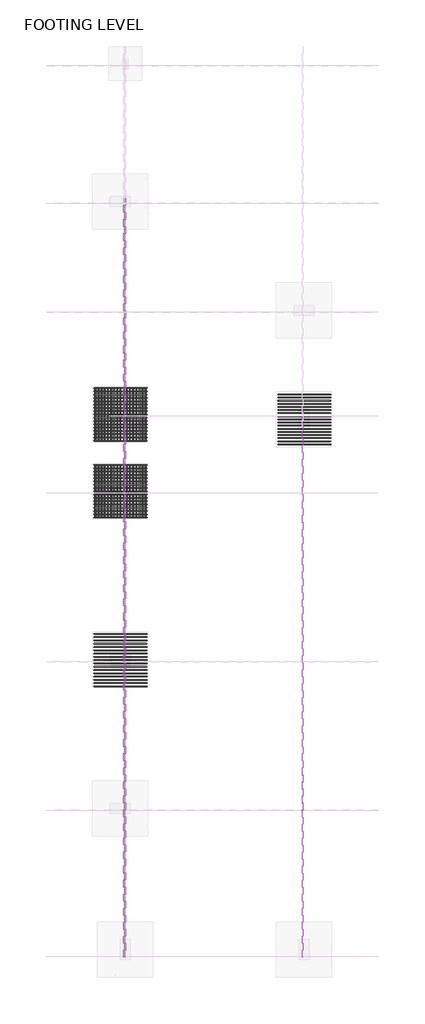
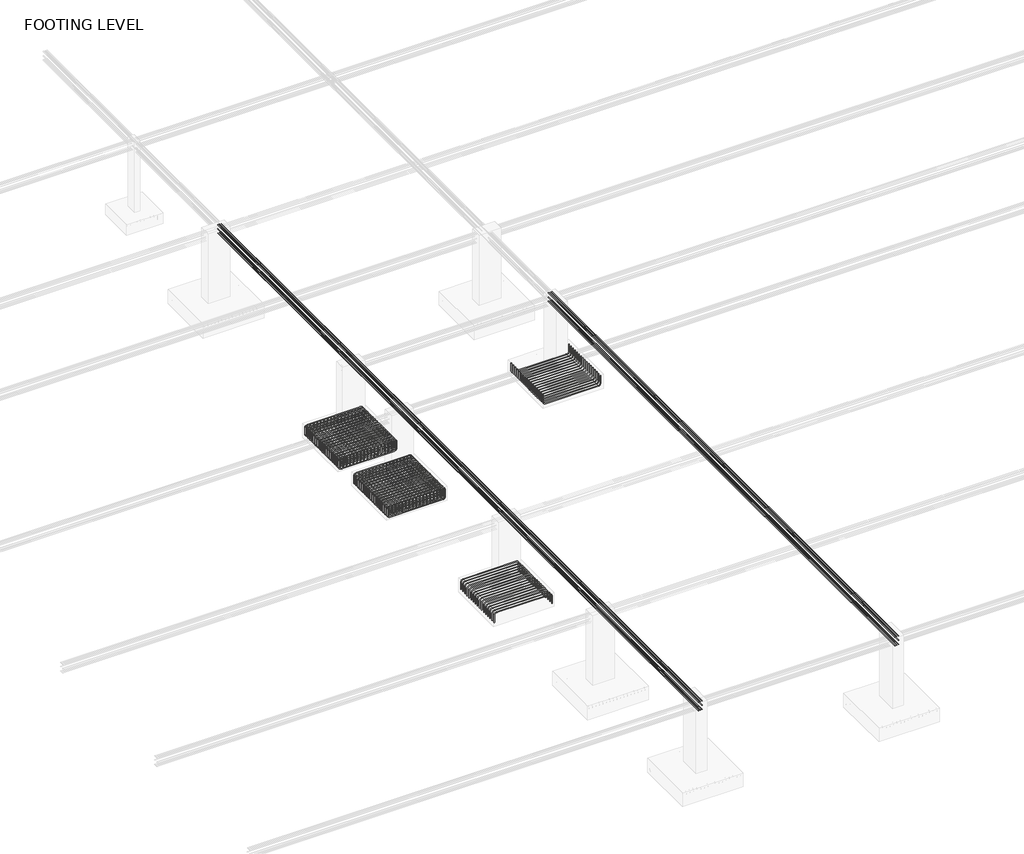
# One storey, part 7 of 19: 16 reinforcing bars.
"""IFC4 building model written with IfcOpenShell, lengths in millimetres."""

from ifc_helpers import new_model, si_unit, point, frame, origin, place, context, project, spatial, polyline, circle_curve, trimmed, segment, composite_curve, source, transform, mapped, element, save
from ifc_brep_helpers import swept_disk

model = new_model("IFC4")

# Units and contexts
model_context = context("Model", 3, world=origin())
ifc_project = project(units=[si_unit("LENGTHUNIT", "METRE", prefix="MILLI")], contexts=[model_context])

# Site, building, storey
site = spatial("IfcSite", under=ifc_project)
building = spatial("IfcBuilding", under=site)
storey = spatial("IfcBuildingStorey", under=building, Name="FOOTING LEVEL", Elevation=-3048.0)

# Reinforcing bars
placement = place(None, origin())
reinforcing_bar_shape = source(origin(), model_context, "Body", "SolidModel", [
    swept_disk(composite_curve([segment(polyline([(10639.8587563, -5025.9516566, -3148.0), (10639.8587563, -5025.9516566, -3470.1)]), True, "CONTINUOUS"), segment(trimmed(circle_curve(frame((10549.6587563, -5025.9516566, -3470.1), z_axis=(0.0, 1.0, 0.0), x_axis=(90.20000000000073, 0.0, 0.0)), 90.2), [point((10639.8587563, -5025.9516566, -3470.1))], [point((10549.6587563, -5025.9516566, -3560.3))], True, "CARTESIAN"), True, "CONTINUOUS"), segment(polyline([(10549.6587563, -5025.9516566, -3560.3), (8355.4587563, -5025.9516566, -3560.3)]), True, "CONTINUOUS"), segment(trimmed(circle_curve(frame((8355.4587563, -5025.9516566, -3470.1), z_axis=(0.0, 1.0, 0.0), x_axis=(0.0, 0.0, -90.20000000000027)), 90.2), [point((8355.4587563, -5025.9516566, -3560.3))], [point((8265.2587563, -5025.9516566, -3470.1))], True, "CARTESIAN"), True, "CONTINUOUS"), segment(polyline([(8265.2587563, -5025.9516566, -3470.1), (8265.2587563, -5025.9516566, -3148.0)]), True, "CONTINUOUS")], self_intersect=False), 12.7),
])
element("IfcReinforcingBar", 1, at=placement, inside=storey, context=model_context, shape_type="MappedRepresentation", body=[
    mapped(reinforcing_bar_shape, transform((0.0, 0.0, 0.0), x_axis=(1.0, 0.0, 0.0), y_axis=(0.0, 1.0, 0.0), z_axis=(0.0, 0.0, 1.0))),
    mapped(reinforcing_bar_shape, transform((0.0, 140.8090411, 0.0), x_axis=(1.0, 0.0, 0.0), y_axis=(0.0, 1.0, 0.0), z_axis=(0.0, 0.0, 1.0))),
    mapped(reinforcing_bar_shape, transform((0.0, 281.6180821, 0.0), x_axis=(1.0, 0.0, 0.0), y_axis=(0.0, 1.0, 0.0), z_axis=(0.0, 0.0, 1.0))),
    mapped(reinforcing_bar_shape, transform((0.0, 422.4271232, 0.0), x_axis=(1.0, 0.0, 0.0), y_axis=(0.0, 1.0, 0.0), z_axis=(0.0, 0.0, 1.0))),
    mapped(reinforcing_bar_shape, transform((0.0, 563.2361643, 0.0), x_axis=(1.0, 0.0, 0.0), y_axis=(0.0, 1.0, 0.0), z_axis=(0.0, 0.0, 1.0))),
    mapped(reinforcing_bar_shape, transform((0.0, 704.0452054, 0.0), x_axis=(1.0, 0.0, 0.0), y_axis=(0.0, 1.0, 0.0), z_axis=(0.0, 0.0, 1.0))),
    mapped(reinforcing_bar_shape, transform((0.0, 844.8542464, 0.0), x_axis=(1.0, 0.0, 0.0), y_axis=(0.0, 1.0, 0.0), z_axis=(0.0, 0.0, 1.0))),
    mapped(reinforcing_bar_shape, transform((0.0, 985.6632875, 0.0), x_axis=(1.0, 0.0, 0.0), y_axis=(0.0, 1.0, 0.0), z_axis=(0.0, 0.0, 1.0))),
    mapped(reinforcing_bar_shape, transform((0.0, 1126.4723286, 0.0), x_axis=(1.0, 0.0, 0.0), y_axis=(0.0, 1.0, 0.0), z_axis=(0.0, 0.0, 1.0))),
    mapped(reinforcing_bar_shape, transform((0.0, 1267.2813697, 0.0), x_axis=(1.0, 0.0, 0.0), y_axis=(0.0, 1.0, 0.0), z_axis=(0.0, 0.0, 1.0))),
    mapped(reinforcing_bar_shape, transform((0.0, 1408.0904107, 0.0), x_axis=(1.0, 0.0, 0.0), y_axis=(0.0, 1.0, 0.0), z_axis=(0.0, 0.0, 1.0))),
    mapped(reinforcing_bar_shape, transform((0.0, 1548.8994518, 0.0), x_axis=(1.0, 0.0, 0.0), y_axis=(0.0, 1.0, 0.0), z_axis=(0.0, 0.0, 1.0))),
    mapped(reinforcing_bar_shape, transform((0.0, 1689.7084929, 0.0), x_axis=(1.0, 0.0, 0.0), y_axis=(0.0, 1.0, 0.0), z_axis=(0.0, 0.0, 1.0))),
    mapped(reinforcing_bar_shape, transform((0.0, 1830.517534, 0.0), x_axis=(1.0, 0.0, 0.0), y_axis=(0.0, 1.0, 0.0), z_axis=(0.0, 0.0, 1.0))),
    mapped(reinforcing_bar_shape, transform((0.0, 1971.326575, 0.0), x_axis=(1.0, 0.0, 0.0), y_axis=(0.0, 1.0, 0.0), z_axis=(0.0, 0.0, 1.0))),
    mapped(reinforcing_bar_shape, transform((0.0, 2112.1356161, 0.0), x_axis=(1.0, 0.0, 0.0), y_axis=(0.0, 1.0, 0.0), z_axis=(0.0, 0.0, 1.0))),
    mapped(reinforcing_bar_shape, transform((0.0, 2252.9446572, 0.0), x_axis=(1.0, 0.0, 0.0), y_axis=(0.0, 1.0, 0.0), z_axis=(0.0, 0.0, 1.0))),
])
reinforcing_bar_2_shape = source(origin(), model_context, "Body", "SolidModel", [
    swept_disk(composite_curve([segment(polyline([(2334.0587563, -13575.4205555, -3523.0), (2334.0587563, -13575.4205555, -3200.9)]), True, "CONTINUOUS"), segment(trimmed(circle_curve(frame((2243.8587563, -13575.4205555, -3200.9), z_axis=(0.0, -1.0, 0.0), x_axis=(90.19999999999982, 0.0, 0.0)), 90.2), [point((2334.0587563, -13575.4205555, -3200.9))], [point((2243.8587563, -13575.4205555, -3110.7))], True, "CARTESIAN"), True, "CONTINUOUS"), segment(polyline([(2243.8587563, -13575.4205555, -3110.7), (49.6587563, -13575.4205555, -3110.7)]), True, "CONTINUOUS"), segment(trimmed(circle_curve(frame((49.6587563, -13575.4205555, -3200.9), z_axis=(0.0, -1.0, 0.0), x_axis=(0.0, 0.0, 90.20000000000027)), 90.2), [point((49.6587563, -13575.4205555, -3110.7))], [point((-40.5412437, -13575.4205555, -3200.9))], True, "CARTESIAN"), True, "CONTINUOUS"), segment(polyline([(-40.5412437, -13575.4205555, -3200.9), (-40.5412437, -13575.4205555, -3523.0)]), True, "CONTINUOUS")], self_intersect=False), 12.7),
])
element("IfcReinforcingBar", 2, at=placement, inside=storey, context=model_context, shape_type="MappedRepresentation", body=[
    mapped(reinforcing_bar_2_shape, transform((0.0, 0.0, 0.0), x_axis=(1.0, 0.0, 0.0), y_axis=(0.0, 1.0, 0.0), z_axis=(0.0, 0.0, 1.0))),
    mapped(reinforcing_bar_2_shape, transform((0.0, -148.4125, 0.0), x_axis=(1.0, 0.0, 0.0), y_axis=(0.0, 1.0, 0.0), z_axis=(0.0, 0.0, 1.0))),
    mapped(reinforcing_bar_2_shape, transform((0.0, -296.825, 0.0), x_axis=(1.0, 0.0, 0.0), y_axis=(0.0, 1.0, 0.0), z_axis=(0.0, 0.0, 1.0))),
    mapped(reinforcing_bar_2_shape, transform((0.0, -445.2375, 0.0), x_axis=(1.0, 0.0, 0.0), y_axis=(0.0, 1.0, 0.0), z_axis=(0.0, 0.0, 1.0))),
    mapped(reinforcing_bar_2_shape, transform((0.0, -593.65, 0.0), x_axis=(1.0, 0.0, 0.0), y_axis=(0.0, 1.0, 0.0), z_axis=(0.0, 0.0, 1.0))),
    mapped(reinforcing_bar_2_shape, transform((0.0, -742.0625, 0.0), x_axis=(1.0, 0.0, 0.0), y_axis=(0.0, 1.0, 0.0), z_axis=(0.0, 0.0, 1.0))),
    mapped(reinforcing_bar_2_shape, transform((0.0, -890.475, 0.0), x_axis=(1.0, 0.0, 0.0), y_axis=(0.0, 1.0, 0.0), z_axis=(0.0, 0.0, 1.0))),
    mapped(reinforcing_bar_2_shape, transform((0.0, -1038.8875, 0.0), x_axis=(1.0, 0.0, 0.0), y_axis=(0.0, 1.0, 0.0), z_axis=(0.0, 0.0, 1.0))),
    mapped(reinforcing_bar_2_shape, transform((0.0, -1187.3, 0.0), x_axis=(1.0, 0.0, 0.0), y_axis=(0.0, 1.0, 0.0), z_axis=(0.0, 0.0, 1.0))),
    mapped(reinforcing_bar_2_shape, transform((0.0, -1335.7125, 0.0), x_axis=(1.0, 0.0, 0.0), y_axis=(0.0, 1.0, 0.0), z_axis=(0.0, 0.0, 1.0))),
    mapped(reinforcing_bar_2_shape, transform((0.0, -1484.125, 0.0), x_axis=(1.0, 0.0, 0.0), y_axis=(0.0, 1.0, 0.0), z_axis=(0.0, 0.0, 1.0))),
    mapped(reinforcing_bar_2_shape, transform((0.0, -1632.5375, 0.0), x_axis=(1.0, 0.0, 0.0), y_axis=(0.0, 1.0, 0.0), z_axis=(0.0, 0.0, 1.0))),
    mapped(reinforcing_bar_2_shape, transform((0.0, -1780.95, 0.0), x_axis=(1.0, 0.0, 0.0), y_axis=(0.0, 1.0, 0.0), z_axis=(0.0, 0.0, 1.0))),
    mapped(reinforcing_bar_2_shape, transform((0.0, -1929.3625, 0.0), x_axis=(1.0, 0.0, 0.0), y_axis=(0.0, 1.0, 0.0), z_axis=(0.0, 0.0, 1.0))),
    mapped(reinforcing_bar_2_shape, transform((0.0, -2077.775, 0.0), x_axis=(1.0, 0.0, 0.0), y_axis=(0.0, 1.0, 0.0), z_axis=(0.0, 0.0, 1.0))),
    mapped(reinforcing_bar_2_shape, transform((0.0, -2226.1875, 0.0), x_axis=(1.0, 0.0, 0.0), y_axis=(0.0, 1.0, 0.0), z_axis=(0.0, 0.0, 1.0))),
    mapped(reinforcing_bar_2_shape, transform((0.0, -2374.6, 0.0), x_axis=(1.0, 0.0, 0.0), y_axis=(0.0, 1.0, 0.0), z_axis=(0.0, 0.0, 1.0))),
])
reinforcing_bar_3_shape = source(origin(), model_context, "Body", "SolidModel", [
    swept_disk(composite_curve([segment(polyline([(25.0276552, -8330.0205555, -3148.0), (25.0276552, -8330.0205555, -3470.1)]), True, "CONTINUOUS"), segment(trimmed(circle_curve(frame((25.0276552, -8239.8205555, -3470.1), z_axis=(1.0, 0.0, 0.0), x_axis=(0.0, -90.19999999999891, 0.0)), 90.2), [point((25.0276552, -8330.0205555, -3470.1))], [point((25.0276552, -8239.8205555, -3560.3))], True, "CARTESIAN"), True, "CONTINUOUS"), segment(polyline([(25.0276552, -8239.8205555, -3560.3), (25.0276552, -6045.6205555, -3560.3)]), True, "CONTINUOUS"), segment(trimmed(circle_curve(frame((25.0276552, -6045.6205555, -3470.1), z_axis=(1.0, 0.0, 0.0), x_axis=(0.0, 0.0, -90.20000000000027)), 90.2), [point((25.0276552, -6045.6205555, -3560.3))], [point((25.0276552, -5955.4205555, -3470.1))], True, "CARTESIAN"), True, "CONTINUOUS"), segment(polyline([(25.0276552, -5955.4205555, -3470.1), (25.0276552, -5955.4205555, -3148.0)]), True, "CONTINUOUS")], self_intersect=False), 12.7),
])
element("IfcReinforcingBar", 3, at=placement, inside=storey, context=model_context, shape_type="MappedRepresentation", body=[
    mapped(reinforcing_bar_3_shape, transform((0.0, 0.0, 0.0), x_axis=(1.0, 0.0, 0.0), y_axis=(0.0, 1.0, 0.0), z_axis=(0.0, 0.0, 1.0))),
    mapped(reinforcing_bar_3_shape, transform((140.8090411, 0.0, 0.0), x_axis=(1.0, 0.0, 0.0), y_axis=(0.0, 1.0, 0.0), z_axis=(0.0, 0.0, 1.0))),
    mapped(reinforcing_bar_3_shape, transform((281.6180821, 0.0, 0.0), x_axis=(1.0, 0.0, 0.0), y_axis=(0.0, 1.0, 0.0), z_axis=(0.0, 0.0, 1.0))),
    mapped(reinforcing_bar_3_shape, transform((422.4271232, 0.0, 0.0), x_axis=(1.0, 0.0, 0.0), y_axis=(0.0, 1.0, 0.0), z_axis=(0.0, 0.0, 1.0))),
    mapped(reinforcing_bar_3_shape, transform((563.2361643, 0.0, 0.0), x_axis=(1.0, 0.0, 0.0), y_axis=(0.0, 1.0, 0.0), z_axis=(0.0, 0.0, 1.0))),
    mapped(reinforcing_bar_3_shape, transform((704.0452054, 0.0, 0.0), x_axis=(1.0, 0.0, 0.0), y_axis=(0.0, 1.0, 0.0), z_axis=(0.0, 0.0, 1.0))),
    mapped(reinforcing_bar_3_shape, transform((844.8542464, 0.0, 0.0), x_axis=(1.0, 0.0, 0.0), y_axis=(0.0, 1.0, 0.0), z_axis=(0.0, 0.0, 1.0))),
    mapped(reinforcing_bar_3_shape, transform((985.6632875, 0.0, 0.0), x_axis=(1.0, 0.0, 0.0), y_axis=(0.0, 1.0, 0.0), z_axis=(0.0, 0.0, 1.0))),
    mapped(reinforcing_bar_3_shape, transform((1126.4723286, 0.0, 0.0), x_axis=(1.0, 0.0, 0.0), y_axis=(0.0, 1.0, 0.0), z_axis=(0.0, 0.0, 1.0))),
    mapped(reinforcing_bar_3_shape, transform((1267.2813697, 0.0, 0.0), x_axis=(1.0, 0.0, 0.0), y_axis=(0.0, 1.0, 0.0), z_axis=(0.0, 0.0, 1.0))),
    mapped(reinforcing_bar_3_shape, transform((1408.0904107, 0.0, 0.0), x_axis=(1.0, 0.0, 0.0), y_axis=(0.0, 1.0, 0.0), z_axis=(0.0, 0.0, 1.0))),
    mapped(reinforcing_bar_3_shape, transform((1548.8994518, 0.0, 0.0), x_axis=(1.0, 0.0, 0.0), y_axis=(0.0, 1.0, 0.0), z_axis=(0.0, 0.0, 1.0))),
    mapped(reinforcing_bar_3_shape, transform((1689.7084929, 0.0, 0.0), x_axis=(1.0, 0.0, 0.0), y_axis=(0.0, 1.0, 0.0), z_axis=(0.0, 0.0, 1.0))),
    mapped(reinforcing_bar_3_shape, transform((1830.517534, 0.0, 0.0), x_axis=(1.0, 0.0, 0.0), y_axis=(0.0, 1.0, 0.0), z_axis=(0.0, 0.0, 1.0))),
    mapped(reinforcing_bar_3_shape, transform((1971.326575, 0.0, 0.0), x_axis=(1.0, 0.0, 0.0), y_axis=(0.0, 1.0, 0.0), z_axis=(0.0, 0.0, 1.0))),
    mapped(reinforcing_bar_3_shape, transform((2112.1356161, 0.0, 0.0), x_axis=(1.0, 0.0, 0.0), y_axis=(0.0, 1.0, 0.0), z_axis=(0.0, 0.0, 1.0))),
    mapped(reinforcing_bar_3_shape, transform((2252.9446572, 0.0, 0.0), x_axis=(1.0, 0.0, 0.0), y_axis=(0.0, 1.0, 0.0), z_axis=(0.0, 0.0, 1.0))),
])
reinforcing_bar_4_shape = source(origin(), model_context, "Body", "SolidModel", [
    swept_disk(composite_curve([segment(polyline([(2300.4197045, -8330.0205555, -3548.0), (2300.4197045, -8330.0205555, -3225.9)]), True, "CONTINUOUS"), segment(trimmed(circle_curve(frame((2300.4197045, -8239.8205555, -3225.9), z_axis=(-1.0, 0.0, 0.0), x_axis=(0.0, -90.19999999999891, 0.0)), 90.2), [point((2300.4197045, -8330.0205555, -3225.9))], [point((2300.4197045, -8239.8205555, -3135.7))], True, "CARTESIAN"), True, "CONTINUOUS"), segment(polyline([(2300.4197045, -8239.8205555, -3135.7), (2300.4197045, -6045.6205555, -3135.7)]), True, "CONTINUOUS"), segment(trimmed(circle_curve(frame((2300.4197045, -6045.6205555, -3225.9), z_axis=(-1.0, 0.0, 0.0), x_axis=(0.0, 0.0, 90.20000000000027)), 90.2), [point((2300.4197045, -6045.6205555, -3135.7))], [point((2300.4197045, -5955.4205555, -3225.9))], True, "CARTESIAN"), True, "CONTINUOUS"), segment(polyline([(2300.4197045, -5955.4205555, -3225.9), (2300.4197045, -5955.4205555, -3548.0)]), True, "CONTINUOUS")], self_intersect=False), 12.7),
])
element("IfcReinforcingBar", 4, at=placement, inside=storey, context=model_context, shape_type="MappedRepresentation", body=[
    mapped(reinforcing_bar_4_shape, transform((0.0, 0.0, 0.0), x_axis=(1.0, 0.0, 0.0), y_axis=(0.0, 1.0, 0.0), z_axis=(0.0, 0.0, 1.0))),
    mapped(reinforcing_bar_4_shape, transform((-143.8496077, 0.0, 0.0), x_axis=(1.0, 0.0, 0.0), y_axis=(0.0, 1.0, 0.0), z_axis=(0.0, 0.0, 1.0))),
    mapped(reinforcing_bar_4_shape, transform((-287.6992155, 0.0, 0.0), x_axis=(1.0, 0.0, 0.0), y_axis=(0.0, 1.0, 0.0), z_axis=(0.0, 0.0, 1.0))),
    mapped(reinforcing_bar_4_shape, transform((-431.5488232, 0.0, 0.0), x_axis=(1.0, 0.0, 0.0), y_axis=(0.0, 1.0, 0.0), z_axis=(0.0, 0.0, 1.0))),
    mapped(reinforcing_bar_4_shape, transform((-575.398431, 0.0, 0.0), x_axis=(1.0, 0.0, 0.0), y_axis=(0.0, 1.0, 0.0), z_axis=(0.0, 0.0, 1.0))),
    mapped(reinforcing_bar_4_shape, transform((-719.2480387, 0.0, 0.0), x_axis=(1.0, 0.0, 0.0), y_axis=(0.0, 1.0, 0.0), z_axis=(0.0, 0.0, 1.0))),
    mapped(reinforcing_bar_4_shape, transform((-863.0976465, 0.0, 0.0), x_axis=(1.0, 0.0, 0.0), y_axis=(0.0, 1.0, 0.0), z_axis=(0.0, 0.0, 1.0))),
    mapped(reinforcing_bar_4_shape, transform((-1006.9472542, 0.0, 0.0), x_axis=(1.0, 0.0, 0.0), y_axis=(0.0, 1.0, 0.0), z_axis=(0.0, 0.0, 1.0))),
    mapped(reinforcing_bar_4_shape, transform((-1150.796862, 0.0, 0.0), x_axis=(1.0, 0.0, 0.0), y_axis=(0.0, 1.0, 0.0), z_axis=(0.0, 0.0, 1.0))),
    mapped(reinforcing_bar_4_shape, transform((-1294.6464697, 0.0, 0.0), x_axis=(1.0, 0.0, 0.0), y_axis=(0.0, 1.0, 0.0), z_axis=(0.0, 0.0, 1.0))),
    mapped(reinforcing_bar_4_shape, transform((-1438.4960775, 0.0, 0.0), x_axis=(1.0, 0.0, 0.0), y_axis=(0.0, 1.0, 0.0), z_axis=(0.0, 0.0, 1.0))),
    mapped(reinforcing_bar_4_shape, transform((-1582.3456852, 0.0, 0.0), x_axis=(1.0, 0.0, 0.0), y_axis=(0.0, 1.0, 0.0), z_axis=(0.0, 0.0, 1.0))),
    mapped(reinforcing_bar_4_shape, transform((-1726.195293, 0.0, 0.0), x_axis=(1.0, 0.0, 0.0), y_axis=(0.0, 1.0, 0.0), z_axis=(0.0, 0.0, 1.0))),
    mapped(reinforcing_bar_4_shape, transform((-1870.0449007, 0.0, 0.0), x_axis=(1.0, 0.0, 0.0), y_axis=(0.0, 1.0, 0.0), z_axis=(0.0, 0.0, 1.0))),
    mapped(reinforcing_bar_4_shape, transform((-2013.8945085, 0.0, 0.0), x_axis=(1.0, 0.0, 0.0), y_axis=(0.0, 1.0, 0.0), z_axis=(0.0, 0.0, 1.0))),
    mapped(reinforcing_bar_4_shape, transform((-2157.7441162, 0.0, 0.0), x_axis=(1.0, 0.0, 0.0), y_axis=(0.0, 1.0, 0.0), z_axis=(0.0, 0.0, 1.0))),
    mapped(reinforcing_bar_4_shape, transform((-2301.5937239, 0.0, 0.0), x_axis=(1.0, 0.0, 0.0), y_axis=(0.0, 1.0, 0.0), z_axis=(0.0, 0.0, 1.0))),
])
reinforcing_bar_5_shape = source(origin(), model_context, "Body", "SolidModel", [
    swept_disk(composite_curve([segment(polyline([(-40.5412437, -5955.4205555, -3173.0), (-40.5412437, -5955.4205555, -3495.1)]), True, "CONTINUOUS"), segment(trimmed(circle_curve(frame((49.6587563, -5955.4205555, -3495.1), z_axis=(0.0, -1.0, 0.0), x_axis=(-90.2, 0.0, 0.0)), 90.2), [point((-40.5412437, -5955.4205555, -3495.1))], [point((49.6587563, -5955.4205555, -3585.3))], True, "CARTESIAN"), True, "CONTINUOUS"), segment(polyline([(49.6587563, -5955.4205555, -3585.3), (2243.8587563, -5955.4205555, -3585.3)]), True, "CONTINUOUS"), segment(trimmed(circle_curve(frame((2243.8587563, -5955.4205555, -3495.1), z_axis=(0.0, -1.0, 0.0), x_axis=(0.0, 0.0, -90.20000000000027)), 90.2), [point((2243.8587563, -5955.4205555, -3585.3))], [point((2334.0587563, -5955.4205555, -3495.1))], True, "CARTESIAN"), True, "CONTINUOUS"), segment(polyline([(2334.0587563, -5955.4205555, -3495.1), (2334.0587563, -5955.4205555, -3173.0)]), True, "CONTINUOUS")], self_intersect=False), 12.7),
])
element("IfcReinforcingBar", 5, at=placement, inside=storey, context=model_context, shape_type="MappedRepresentation", body=[
    mapped(reinforcing_bar_5_shape, transform((0.0, 0.0, 0.0), x_axis=(1.0, 0.0, 0.0), y_axis=(0.0, 1.0, 0.0), z_axis=(0.0, 0.0, 1.0))),
    mapped(reinforcing_bar_5_shape, transform((0.0, -148.4125, 0.0), x_axis=(1.0, 0.0, 0.0), y_axis=(0.0, 1.0, 0.0), z_axis=(0.0, 0.0, 1.0))),
    mapped(reinforcing_bar_5_shape, transform((0.0, -296.825, 0.0), x_axis=(1.0, 0.0, 0.0), y_axis=(0.0, 1.0, 0.0), z_axis=(0.0, 0.0, 1.0))),
    mapped(reinforcing_bar_5_shape, transform((0.0, -445.2375, 0.0), x_axis=(1.0, 0.0, 0.0), y_axis=(0.0, 1.0, 0.0), z_axis=(0.0, 0.0, 1.0))),
    mapped(reinforcing_bar_5_shape, transform((0.0, -593.65, 0.0), x_axis=(1.0, 0.0, 0.0), y_axis=(0.0, 1.0, 0.0), z_axis=(0.0, 0.0, 1.0))),
    mapped(reinforcing_bar_5_shape, transform((0.0, -742.0625, 0.0), x_axis=(1.0, 0.0, 0.0), y_axis=(0.0, 1.0, 0.0), z_axis=(0.0, 0.0, 1.0))),
    mapped(reinforcing_bar_5_shape, transform((0.0, -890.475, 0.0), x_axis=(1.0, 0.0, 0.0), y_axis=(0.0, 1.0, 0.0), z_axis=(0.0, 0.0, 1.0))),
    mapped(reinforcing_bar_5_shape, transform((0.0, -1038.8875, 0.0), x_axis=(1.0, 0.0, 0.0), y_axis=(0.0, 1.0, 0.0), z_axis=(0.0, 0.0, 1.0))),
    mapped(reinforcing_bar_5_shape, transform((0.0, -1187.3, 0.0), x_axis=(1.0, 0.0, 0.0), y_axis=(0.0, 1.0, 0.0), z_axis=(0.0, 0.0, 1.0))),
    mapped(reinforcing_bar_5_shape, transform((0.0, -1335.7125, 0.0), x_axis=(1.0, 0.0, 0.0), y_axis=(0.0, 1.0, 0.0), z_axis=(0.0, 0.0, 1.0))),
    mapped(reinforcing_bar_5_shape, transform((0.0, -1484.125, 0.0), x_axis=(1.0, 0.0, 0.0), y_axis=(0.0, 1.0, 0.0), z_axis=(0.0, 0.0, 1.0))),
    mapped(reinforcing_bar_5_shape, transform((0.0, -1632.5375, 0.0), x_axis=(1.0, 0.0, 0.0), y_axis=(0.0, 1.0, 0.0), z_axis=(0.0, 0.0, 1.0))),
    mapped(reinforcing_bar_5_shape, transform((0.0, -1780.95, 0.0), x_axis=(1.0, 0.0, 0.0), y_axis=(0.0, 1.0, 0.0), z_axis=(0.0, 0.0, 1.0))),
    mapped(reinforcing_bar_5_shape, transform((0.0, -1929.3625, 0.0), x_axis=(1.0, 0.0, 0.0), y_axis=(0.0, 1.0, 0.0), z_axis=(0.0, 0.0, 1.0))),
    mapped(reinforcing_bar_5_shape, transform((0.0, -2077.775, 0.0), x_axis=(1.0, 0.0, 0.0), y_axis=(0.0, 1.0, 0.0), z_axis=(0.0, 0.0, 1.0))),
    mapped(reinforcing_bar_5_shape, transform((0.0, -2226.1875, 0.0), x_axis=(1.0, 0.0, 0.0), y_axis=(0.0, 1.0, 0.0), z_axis=(0.0, 0.0, 1.0))),
    mapped(reinforcing_bar_5_shape, transform((0.0, -2374.6, 0.0), x_axis=(1.0, 0.0, 0.0), y_axis=(0.0, 1.0, 0.0), z_axis=(0.0, 0.0, 1.0))),
])
reinforcing_bar_6_shape = source(origin(), model_context, "Body", "SolidModel", [
    swept_disk(composite_curve([segment(polyline([(2334.0587563, -5955.4205555, -3523.0), (2334.0587563, -5955.4205555, -3200.9)]), True, "CONTINUOUS"), segment(trimmed(circle_curve(frame((2243.8587563, -5955.4205555, -3200.9), z_axis=(0.0, -1.0, 0.0), x_axis=(90.19999999999982, 0.0, 0.0)), 90.2), [point((2334.0587563, -5955.4205555, -3200.9))], [point((2243.8587563, -5955.4205555, -3110.7))], True, "CARTESIAN"), True, "CONTINUOUS"), segment(polyline([(2243.8587563, -5955.4205555, -3110.7), (49.6587563, -5955.4205555, -3110.7)]), True, "CONTINUOUS"), segment(trimmed(circle_curve(frame((49.6587563, -5955.4205555, -3200.9), z_axis=(0.0, -1.0, 0.0), x_axis=(0.0, 0.0, 90.20000000000027)), 90.2), [point((49.6587563, -5955.4205555, -3110.7))], [point((-40.5412437, -5955.4205555, -3200.9))], True, "CARTESIAN"), True, "CONTINUOUS"), segment(polyline([(-40.5412437, -5955.4205555, -3200.9), (-40.5412437, -5955.4205555, -3523.0)]), True, "CONTINUOUS")], self_intersect=False), 12.7),
])
element("IfcReinforcingBar", 6, at=placement, inside=storey, context=model_context, shape_type="MappedRepresentation", body=[
    mapped(reinforcing_bar_6_shape, transform((0.0, 0.0, 0.0), x_axis=(1.0, 0.0, 0.0), y_axis=(0.0, 1.0, 0.0), z_axis=(0.0, 0.0, 1.0))),
    mapped(reinforcing_bar_6_shape, transform((0.0, -148.4125, 0.0), x_axis=(1.0, 0.0, 0.0), y_axis=(0.0, 1.0, 0.0), z_axis=(0.0, 0.0, 1.0))),
    mapped(reinforcing_bar_6_shape, transform((0.0, -296.825, 0.0), x_axis=(1.0, 0.0, 0.0), y_axis=(0.0, 1.0, 0.0), z_axis=(0.0, 0.0, 1.0))),
    mapped(reinforcing_bar_6_shape, transform((0.0, -445.2375, 0.0), x_axis=(1.0, 0.0, 0.0), y_axis=(0.0, 1.0, 0.0), z_axis=(0.0, 0.0, 1.0))),
    mapped(reinforcing_bar_6_shape, transform((0.0, -593.65, 0.0), x_axis=(1.0, 0.0, 0.0), y_axis=(0.0, 1.0, 0.0), z_axis=(0.0, 0.0, 1.0))),
    mapped(reinforcing_bar_6_shape, transform((0.0, -742.0625, 0.0), x_axis=(1.0, 0.0, 0.0), y_axis=(0.0, 1.0, 0.0), z_axis=(0.0, 0.0, 1.0))),
    mapped(reinforcing_bar_6_shape, transform((0.0, -890.475, 0.0), x_axis=(1.0, 0.0, 0.0), y_axis=(0.0, 1.0, 0.0), z_axis=(0.0, 0.0, 1.0))),
    mapped(reinforcing_bar_6_shape, transform((0.0, -1038.8875, 0.0), x_axis=(1.0, 0.0, 0.0), y_axis=(0.0, 1.0, 0.0), z_axis=(0.0, 0.0, 1.0))),
    mapped(reinforcing_bar_6_shape, transform((0.0, -1187.3, 0.0), x_axis=(1.0, 0.0, 0.0), y_axis=(0.0, 1.0, 0.0), z_axis=(0.0, 0.0, 1.0))),
    mapped(reinforcing_bar_6_shape, transform((0.0, -1335.7125, 0.0), x_axis=(1.0, 0.0, 0.0), y_axis=(0.0, 1.0, 0.0), z_axis=(0.0, 0.0, 1.0))),
    mapped(reinforcing_bar_6_shape, transform((0.0, -1484.125, 0.0), x_axis=(1.0, 0.0, 0.0), y_axis=(0.0, 1.0, 0.0), z_axis=(0.0, 0.0, 1.0))),
    mapped(reinforcing_bar_6_shape, transform((0.0, -1632.5375, 0.0), x_axis=(1.0, 0.0, 0.0), y_axis=(0.0, 1.0, 0.0), z_axis=(0.0, 0.0, 1.0))),
    mapped(reinforcing_bar_6_shape, transform((0.0, -1780.95, 0.0), x_axis=(1.0, 0.0, 0.0), y_axis=(0.0, 1.0, 0.0), z_axis=(0.0, 0.0, 1.0))),
    mapped(reinforcing_bar_6_shape, transform((0.0, -1929.3625, 0.0), x_axis=(1.0, 0.0, 0.0), y_axis=(0.0, 1.0, 0.0), z_axis=(0.0, 0.0, 1.0))),
    mapped(reinforcing_bar_6_shape, transform((0.0, -2077.775, 0.0), x_axis=(1.0, 0.0, 0.0), y_axis=(0.0, 1.0, 0.0), z_axis=(0.0, 0.0, 1.0))),
    mapped(reinforcing_bar_6_shape, transform((0.0, -2226.1875, 0.0), x_axis=(1.0, 0.0, 0.0), y_axis=(0.0, 1.0, 0.0), z_axis=(0.0, 0.0, 1.0))),
    mapped(reinforcing_bar_6_shape, transform((0.0, -2374.6, 0.0), x_axis=(1.0, 0.0, 0.0), y_axis=(0.0, 1.0, 0.0), z_axis=(0.0, 0.0, 1.0))),
])
reinforcing_bar_7_shape = source(origin(), model_context, "Body", "SolidModel", [
    swept_disk(composite_curve([segment(polyline([(25.0276552, -4862.9205555, -3148.0), (25.0276552, -4862.9205555, -3470.1)]), True, "CONTINUOUS"), segment(trimmed(circle_curve(frame((25.0276552, -4772.7205555, -3470.1), z_axis=(1.0, 0.0, 0.0), x_axis=(0.0, -90.19999999999982, 0.0)), 90.2), [point((25.0276552, -4862.9205555, -3470.1))], [point((25.0276552, -4772.7205555, -3560.3))], True, "CARTESIAN"), True, "CONTINUOUS"), segment(polyline([(25.0276552, -4772.7205555, -3560.3), (25.0276552, -2578.5205555, -3560.3)]), True, "CONTINUOUS"), segment(trimmed(circle_curve(frame((25.0276552, -2578.5205555, -3470.1), z_axis=(1.0, 0.0, 0.0), x_axis=(0.0, 0.0, -90.20000000000027)), 90.2), [point((25.0276552, -2578.5205555, -3560.3))], [point((25.0276552, -2488.3205555, -3470.1))], True, "CARTESIAN"), True, "CONTINUOUS"), segment(polyline([(25.0276552, -2488.3205555, -3470.1), (25.0276552, -2488.3205555, -3148.0)]), True, "CONTINUOUS")], self_intersect=False), 12.7),
])
element("IfcReinforcingBar", 7, at=placement, inside=storey, context=model_context, shape_type="MappedRepresentation", body=[
    mapped(reinforcing_bar_7_shape, transform((0.0, 0.0, 0.0), x_axis=(1.0, 0.0, 0.0), y_axis=(0.0, 1.0, 0.0), z_axis=(0.0, 0.0, 1.0))),
    mapped(reinforcing_bar_7_shape, transform((140.8090411, 0.0, 0.0), x_axis=(1.0, 0.0, 0.0), y_axis=(0.0, 1.0, 0.0), z_axis=(0.0, 0.0, 1.0))),
    mapped(reinforcing_bar_7_shape, transform((281.6180821, 0.0, 0.0), x_axis=(1.0, 0.0, 0.0), y_axis=(0.0, 1.0, 0.0), z_axis=(0.0, 0.0, 1.0))),
    mapped(reinforcing_bar_7_shape, transform((422.4271232, 0.0, 0.0), x_axis=(1.0, 0.0, 0.0), y_axis=(0.0, 1.0, 0.0), z_axis=(0.0, 0.0, 1.0))),
    mapped(reinforcing_bar_7_shape, transform((563.2361643, 0.0, 0.0), x_axis=(1.0, 0.0, 0.0), y_axis=(0.0, 1.0, 0.0), z_axis=(0.0, 0.0, 1.0))),
    mapped(reinforcing_bar_7_shape, transform((704.0452054, 0.0, 0.0), x_axis=(1.0, 0.0, 0.0), y_axis=(0.0, 1.0, 0.0), z_axis=(0.0, 0.0, 1.0))),
    mapped(reinforcing_bar_7_shape, transform((844.8542464, 0.0, 0.0), x_axis=(1.0, 0.0, 0.0), y_axis=(0.0, 1.0, 0.0), z_axis=(0.0, 0.0, 1.0))),
    mapped(reinforcing_bar_7_shape, transform((985.6632875, 0.0, 0.0), x_axis=(1.0, 0.0, 0.0), y_axis=(0.0, 1.0, 0.0), z_axis=(0.0, 0.0, 1.0))),
    mapped(reinforcing_bar_7_shape, transform((1126.4723286, 0.0, 0.0), x_axis=(1.0, 0.0, 0.0), y_axis=(0.0, 1.0, 0.0), z_axis=(0.0, 0.0, 1.0))),
    mapped(reinforcing_bar_7_shape, transform((1267.2813697, 0.0, 0.0), x_axis=(1.0, 0.0, 0.0), y_axis=(0.0, 1.0, 0.0), z_axis=(0.0, 0.0, 1.0))),
    mapped(reinforcing_bar_7_shape, transform((1408.0904107, 0.0, 0.0), x_axis=(1.0, 0.0, 0.0), y_axis=(0.0, 1.0, 0.0), z_axis=(0.0, 0.0, 1.0))),
    mapped(reinforcing_bar_7_shape, transform((1548.8994518, 0.0, 0.0), x_axis=(1.0, 0.0, 0.0), y_axis=(0.0, 1.0, 0.0), z_axis=(0.0, 0.0, 1.0))),
    mapped(reinforcing_bar_7_shape, transform((1689.7084929, 0.0, 0.0), x_axis=(1.0, 0.0, 0.0), y_axis=(0.0, 1.0, 0.0), z_axis=(0.0, 0.0, 1.0))),
    mapped(reinforcing_bar_7_shape, transform((1830.517534, 0.0, 0.0), x_axis=(1.0, 0.0, 0.0), y_axis=(0.0, 1.0, 0.0), z_axis=(0.0, 0.0, 1.0))),
    mapped(reinforcing_bar_7_shape, transform((1971.326575, 0.0, 0.0), x_axis=(1.0, 0.0, 0.0), y_axis=(0.0, 1.0, 0.0), z_axis=(0.0, 0.0, 1.0))),
    mapped(reinforcing_bar_7_shape, transform((2112.1356161, 0.0, 0.0), x_axis=(1.0, 0.0, 0.0), y_axis=(0.0, 1.0, 0.0), z_axis=(0.0, 0.0, 1.0))),
    mapped(reinforcing_bar_7_shape, transform((2252.9446572, 0.0, 0.0), x_axis=(1.0, 0.0, 0.0), y_axis=(0.0, 1.0, 0.0), z_axis=(0.0, 0.0, 1.0))),
])
reinforcing_bar_8_shape = source(origin(), model_context, "Body", "SolidModel", [
    swept_disk(composite_curve([segment(polyline([(2300.4197045, -4862.9205555, -3548.0), (2300.4197045, -4862.9205555, -3225.9)]), True, "CONTINUOUS"), segment(trimmed(circle_curve(frame((2300.4197045, -4772.7205555, -3225.9), z_axis=(-1.0, 0.0, 0.0), x_axis=(0.0, -90.19999999999982, 0.0)), 90.2), [point((2300.4197045, -4862.9205555, -3225.9))], [point((2300.4197045, -4772.7205555, -3135.7))], True, "CARTESIAN"), True, "CONTINUOUS"), segment(polyline([(2300.4197045, -4772.7205555, -3135.7), (2300.4197045, -2578.5205555, -3135.7)]), True, "CONTINUOUS"), segment(trimmed(circle_curve(frame((2300.4197045, -2578.5205555, -3225.9), z_axis=(-1.0, 0.0, 0.0), x_axis=(0.0, 0.0, 90.20000000000027)), 90.2), [point((2300.4197045, -2578.5205555, -3135.7))], [point((2300.4197045, -2488.3205555, -3225.9))], True, "CARTESIAN"), True, "CONTINUOUS"), segment(polyline([(2300.4197045, -2488.3205555, -3225.9), (2300.4197045, -2488.3205555, -3548.0)]), True, "CONTINUOUS")], self_intersect=False), 12.7),
])
element("IfcReinforcingBar", 8, at=placement, inside=storey, context=model_context, shape_type="MappedRepresentation", body=[
    mapped(reinforcing_bar_8_shape, transform((0.0, 0.0, 0.0), x_axis=(1.0, 0.0, 0.0), y_axis=(0.0, 1.0, 0.0), z_axis=(0.0, 0.0, 1.0))),
    mapped(reinforcing_bar_8_shape, transform((-143.8496077, 0.0, 0.0), x_axis=(1.0, 0.0, 0.0), y_axis=(0.0, 1.0, 0.0), z_axis=(0.0, 0.0, 1.0))),
    mapped(reinforcing_bar_8_shape, transform((-287.6992155, 0.0, 0.0), x_axis=(1.0, 0.0, 0.0), y_axis=(0.0, 1.0, 0.0), z_axis=(0.0, 0.0, 1.0))),
    mapped(reinforcing_bar_8_shape, transform((-431.5488232, 0.0, 0.0), x_axis=(1.0, 0.0, 0.0), y_axis=(0.0, 1.0, 0.0), z_axis=(0.0, 0.0, 1.0))),
    mapped(reinforcing_bar_8_shape, transform((-575.398431, 0.0, 0.0), x_axis=(1.0, 0.0, 0.0), y_axis=(0.0, 1.0, 0.0), z_axis=(0.0, 0.0, 1.0))),
    mapped(reinforcing_bar_8_shape, transform((-719.2480387, 0.0, 0.0), x_axis=(1.0, 0.0, 0.0), y_axis=(0.0, 1.0, 0.0), z_axis=(0.0, 0.0, 1.0))),
    mapped(reinforcing_bar_8_shape, transform((-863.0976465, 0.0, 0.0), x_axis=(1.0, 0.0, 0.0), y_axis=(0.0, 1.0, 0.0), z_axis=(0.0, 0.0, 1.0))),
    mapped(reinforcing_bar_8_shape, transform((-1006.9472542, 0.0, 0.0), x_axis=(1.0, 0.0, 0.0), y_axis=(0.0, 1.0, 0.0), z_axis=(0.0, 0.0, 1.0))),
    mapped(reinforcing_bar_8_shape, transform((-1150.796862, 0.0, 0.0), x_axis=(1.0, 0.0, 0.0), y_axis=(0.0, 1.0, 0.0), z_axis=(0.0, 0.0, 1.0))),
    mapped(reinforcing_bar_8_shape, transform((-1294.6464697, 0.0, 0.0), x_axis=(1.0, 0.0, 0.0), y_axis=(0.0, 1.0, 0.0), z_axis=(0.0, 0.0, 1.0))),
    mapped(reinforcing_bar_8_shape, transform((-1438.4960775, 0.0, 0.0), x_axis=(1.0, 0.0, 0.0), y_axis=(0.0, 1.0, 0.0), z_axis=(0.0, 0.0, 1.0))),
    mapped(reinforcing_bar_8_shape, transform((-1582.3456852, 0.0, 0.0), x_axis=(1.0, 0.0, 0.0), y_axis=(0.0, 1.0, 0.0), z_axis=(0.0, 0.0, 1.0))),
    mapped(reinforcing_bar_8_shape, transform((-1726.195293, 0.0, 0.0), x_axis=(1.0, 0.0, 0.0), y_axis=(0.0, 1.0, 0.0), z_axis=(0.0, 0.0, 1.0))),
    mapped(reinforcing_bar_8_shape, transform((-1870.0449007, 0.0, 0.0), x_axis=(1.0, 0.0, 0.0), y_axis=(0.0, 1.0, 0.0), z_axis=(0.0, 0.0, 1.0))),
    mapped(reinforcing_bar_8_shape, transform((-2013.8945085, 0.0, 0.0), x_axis=(1.0, 0.0, 0.0), y_axis=(0.0, 1.0, 0.0), z_axis=(0.0, 0.0, 1.0))),
    mapped(reinforcing_bar_8_shape, transform((-2157.7441162, 0.0, 0.0), x_axis=(1.0, 0.0, 0.0), y_axis=(0.0, 1.0, 0.0), z_axis=(0.0, 0.0, 1.0))),
    mapped(reinforcing_bar_8_shape, transform((-2301.5937239, 0.0, 0.0), x_axis=(1.0, 0.0, 0.0), y_axis=(0.0, 1.0, 0.0), z_axis=(0.0, 0.0, 1.0))),
])
reinforcing_bar_9_shape = source(origin(), model_context, "Body", "SolidModel", [
    swept_disk(composite_curve([segment(polyline([(-40.5412437, -2488.3205555, -3173.0), (-40.5412437, -2488.3205555, -3495.1)]), True, "CONTINUOUS"), segment(trimmed(circle_curve(frame((49.6587563, -2488.3205555, -3495.1), z_axis=(0.0, -1.0, 0.0), x_axis=(-90.2, 0.0, 0.0)), 90.2), [point((-40.5412437, -2488.3205555, -3495.1))], [point((49.6587563, -2488.3205555, -3585.3))], True, "CARTESIAN"), True, "CONTINUOUS"), segment(polyline([(49.6587563, -2488.3205555, -3585.3), (2243.8587563, -2488.3205555, -3585.3)]), True, "CONTINUOUS"), segment(trimmed(circle_curve(frame((2243.8587563, -2488.3205555, -3495.1), z_axis=(0.0, -1.0, 0.0), x_axis=(0.0, 0.0, -90.20000000000027)), 90.2), [point((2243.8587563, -2488.3205555, -3585.3))], [point((2334.0587563, -2488.3205555, -3495.1))], True, "CARTESIAN"), True, "CONTINUOUS"), segment(polyline([(2334.0587563, -2488.3205555, -3495.1), (2334.0587563, -2488.3205555, -3173.0)]), True, "CONTINUOUS")], self_intersect=False), 12.7),
])
element("IfcReinforcingBar", 9, at=placement, inside=storey, context=model_context, shape_type="MappedRepresentation", body=[
    mapped(reinforcing_bar_9_shape, transform((0.0, 0.0, 0.0), x_axis=(1.0, 0.0, 0.0), y_axis=(0.0, 1.0, 0.0), z_axis=(0.0, 0.0, 1.0))),
    mapped(reinforcing_bar_9_shape, transform((0.0, -148.4125, 0.0), x_axis=(1.0, 0.0, 0.0), y_axis=(0.0, 1.0, 0.0), z_axis=(0.0, 0.0, 1.0))),
    mapped(reinforcing_bar_9_shape, transform((0.0, -296.825, 0.0), x_axis=(1.0, 0.0, 0.0), y_axis=(0.0, 1.0, 0.0), z_axis=(0.0, 0.0, 1.0))),
    mapped(reinforcing_bar_9_shape, transform((0.0, -445.2375, 0.0), x_axis=(1.0, 0.0, 0.0), y_axis=(0.0, 1.0, 0.0), z_axis=(0.0, 0.0, 1.0))),
    mapped(reinforcing_bar_9_shape, transform((0.0, -593.65, 0.0), x_axis=(1.0, 0.0, 0.0), y_axis=(0.0, 1.0, 0.0), z_axis=(0.0, 0.0, 1.0))),
    mapped(reinforcing_bar_9_shape, transform((0.0, -742.0625, 0.0), x_axis=(1.0, 0.0, 0.0), y_axis=(0.0, 1.0, 0.0), z_axis=(0.0, 0.0, 1.0))),
    mapped(reinforcing_bar_9_shape, transform((0.0, -890.475, 0.0), x_axis=(1.0, 0.0, 0.0), y_axis=(0.0, 1.0, 0.0), z_axis=(0.0, 0.0, 1.0))),
    mapped(reinforcing_bar_9_shape, transform((0.0, -1038.8875, 0.0), x_axis=(1.0, 0.0, 0.0), y_axis=(0.0, 1.0, 0.0), z_axis=(0.0, 0.0, 1.0))),
    mapped(reinforcing_bar_9_shape, transform((0.0, -1187.3, 0.0), x_axis=(1.0, 0.0, 0.0), y_axis=(0.0, 1.0, 0.0), z_axis=(0.0, 0.0, 1.0))),
    mapped(reinforcing_bar_9_shape, transform((0.0, -1335.7125, 0.0), x_axis=(1.0, 0.0, 0.0), y_axis=(0.0, 1.0, 0.0), z_axis=(0.0, 0.0, 1.0))),
    mapped(reinforcing_bar_9_shape, transform((0.0, -1484.125, 0.0), x_axis=(1.0, 0.0, 0.0), y_axis=(0.0, 1.0, 0.0), z_axis=(0.0, 0.0, 1.0))),
    mapped(reinforcing_bar_9_shape, transform((0.0, -1632.5375, 0.0), x_axis=(1.0, 0.0, 0.0), y_axis=(0.0, 1.0, 0.0), z_axis=(0.0, 0.0, 1.0))),
    mapped(reinforcing_bar_9_shape, transform((0.0, -1780.95, 0.0), x_axis=(1.0, 0.0, 0.0), y_axis=(0.0, 1.0, 0.0), z_axis=(0.0, 0.0, 1.0))),
    mapped(reinforcing_bar_9_shape, transform((0.0, -1929.3625, 0.0), x_axis=(1.0, 0.0, 0.0), y_axis=(0.0, 1.0, 0.0), z_axis=(0.0, 0.0, 1.0))),
    mapped(reinforcing_bar_9_shape, transform((0.0, -2077.775, 0.0), x_axis=(1.0, 0.0, 0.0), y_axis=(0.0, 1.0, 0.0), z_axis=(0.0, 0.0, 1.0))),
    mapped(reinforcing_bar_9_shape, transform((0.0, -2226.1875, 0.0), x_axis=(1.0, 0.0, 0.0), y_axis=(0.0, 1.0, 0.0), z_axis=(0.0, 0.0, 1.0))),
    mapped(reinforcing_bar_9_shape, transform((0.0, -2374.6, 0.0), x_axis=(1.0, 0.0, 0.0), y_axis=(0.0, 1.0, 0.0), z_axis=(0.0, 0.0, 1.0))),
])
reinforcing_bar_10_shape = source(origin(), model_context, "Body", "SolidModel", [
    swept_disk(composite_curve([segment(polyline([(2334.0587563, -2488.3205555, -3523.0), (2334.0587563, -2488.3205555, -3200.9)]), True, "CONTINUOUS"), segment(trimmed(circle_curve(frame((2243.8587563, -2488.3205555, -3200.9), z_axis=(0.0, -1.0, 0.0), x_axis=(90.19999999999982, 0.0, 0.0)), 90.2), [point((2334.0587563, -2488.3205555, -3200.9))], [point((2243.8587563, -2488.3205555, -3110.7))], True, "CARTESIAN"), True, "CONTINUOUS"), segment(polyline([(2243.8587563, -2488.3205555, -3110.7), (49.6587563, -2488.3205555, -3110.7)]), True, "CONTINUOUS"), segment(trimmed(circle_curve(frame((49.6587563, -2488.3205555, -3200.9), z_axis=(0.0, -1.0, 0.0), x_axis=(0.0, 0.0, 90.20000000000027)), 90.2), [point((49.6587563, -2488.3205555, -3110.7))], [point((-40.5412437, -2488.3205555, -3200.9))], True, "CARTESIAN"), True, "CONTINUOUS"), segment(polyline([(-40.5412437, -2488.3205555, -3200.9), (-40.5412437, -2488.3205555, -3523.0)]), True, "CONTINUOUS")], self_intersect=False), 12.7),
])
element("IfcReinforcingBar", 10, at=placement, inside=storey, context=model_context, shape_type="MappedRepresentation", body=[
    mapped(reinforcing_bar_10_shape, transform((0.0, 0.0, 0.0), x_axis=(1.0, 0.0, 0.0), y_axis=(0.0, 1.0, 0.0), z_axis=(0.0, 0.0, 1.0))),
    mapped(reinforcing_bar_10_shape, transform((0.0, -148.4125, 0.0), x_axis=(1.0, 0.0, 0.0), y_axis=(0.0, 1.0, 0.0), z_axis=(0.0, 0.0, 1.0))),
    mapped(reinforcing_bar_10_shape, transform((0.0, -296.825, 0.0), x_axis=(1.0, 0.0, 0.0), y_axis=(0.0, 1.0, 0.0), z_axis=(0.0, 0.0, 1.0))),
    mapped(reinforcing_bar_10_shape, transform((0.0, -445.2375, 0.0), x_axis=(1.0, 0.0, 0.0), y_axis=(0.0, 1.0, 0.0), z_axis=(0.0, 0.0, 1.0))),
    mapped(reinforcing_bar_10_shape, transform((0.0, -593.65, 0.0), x_axis=(1.0, 0.0, 0.0), y_axis=(0.0, 1.0, 0.0), z_axis=(0.0, 0.0, 1.0))),
    mapped(reinforcing_bar_10_shape, transform((0.0, -742.0625, 0.0), x_axis=(1.0, 0.0, 0.0), y_axis=(0.0, 1.0, 0.0), z_axis=(0.0, 0.0, 1.0))),
    mapped(reinforcing_bar_10_shape, transform((0.0, -890.475, 0.0), x_axis=(1.0, 0.0, 0.0), y_axis=(0.0, 1.0, 0.0), z_axis=(0.0, 0.0, 1.0))),
    mapped(reinforcing_bar_10_shape, transform((0.0, -1038.8875, 0.0), x_axis=(1.0, 0.0, 0.0), y_axis=(0.0, 1.0, 0.0), z_axis=(0.0, 0.0, 1.0))),
    mapped(reinforcing_bar_10_shape, transform((0.0, -1187.3, 0.0), x_axis=(1.0, 0.0, 0.0), y_axis=(0.0, 1.0, 0.0), z_axis=(0.0, 0.0, 1.0))),
    mapped(reinforcing_bar_10_shape, transform((0.0, -1335.7125, 0.0), x_axis=(1.0, 0.0, 0.0), y_axis=(0.0, 1.0, 0.0), z_axis=(0.0, 0.0, 1.0))),
    mapped(reinforcing_bar_10_shape, transform((0.0, -1484.125, 0.0), x_axis=(1.0, 0.0, 0.0), y_axis=(0.0, 1.0, 0.0), z_axis=(0.0, 0.0, 1.0))),
    mapped(reinforcing_bar_10_shape, transform((0.0, -1632.5375, 0.0), x_axis=(1.0, 0.0, 0.0), y_axis=(0.0, 1.0, 0.0), z_axis=(0.0, 0.0, 1.0))),
    mapped(reinforcing_bar_10_shape, transform((0.0, -1780.95, 0.0), x_axis=(1.0, 0.0, 0.0), y_axis=(0.0, 1.0, 0.0), z_axis=(0.0, 0.0, 1.0))),
    mapped(reinforcing_bar_10_shape, transform((0.0, -1929.3625, 0.0), x_axis=(1.0, 0.0, 0.0), y_axis=(0.0, 1.0, 0.0), z_axis=(0.0, 0.0, 1.0))),
    mapped(reinforcing_bar_10_shape, transform((0.0, -2077.775, 0.0), x_axis=(1.0, 0.0, 0.0), y_axis=(0.0, 1.0, 0.0), z_axis=(0.0, 0.0, 1.0))),
    mapped(reinforcing_bar_10_shape, transform((0.0, -2226.1875, 0.0), x_axis=(1.0, 0.0, 0.0), y_axis=(0.0, 1.0, 0.0), z_axis=(0.0, 0.0, 1.0))),
    mapped(reinforcing_bar_10_shape, transform((0.0, -2374.6, 0.0), x_axis=(1.0, 0.0, 0.0), y_axis=(0.0, 1.0, 0.0), z_axis=(0.0, 0.0, 1.0))),
])
reinforcing_bar_11_shape = source(origin(), model_context, "Body", "SolidModel", [
    swept_disk(composite_curve([segment(polyline([(9382.7381195, -3487.0205555, -412.7206367), (9382.7381195, -28174.6911496, -412.7206367)]), True, "CONTINUOUS")], self_intersect=False), 7.95),
])
element("IfcReinforcingBar", 11, at=placement, inside=storey, context=model_context, shape_type="MappedRepresentation", body=[
    mapped(reinforcing_bar_11_shape, transform((0.0, 0.0, 0.0), x_axis=(1.0, 0.0, 0.0), y_axis=(0.0, 1.0, 0.0), z_axis=(0.0, 0.0, 1.0))),
    mapped(reinforcing_bar_11_shape, transform((69.8206367, 0.0, 0.0), x_axis=(1.0, 0.0, 0.0), y_axis=(0.0, 1.0, 0.0), z_axis=(0.0, 0.0, 1.0))),
    mapped(reinforcing_bar_11_shape, transform((139.6412734, 0.0, 0.0), x_axis=(1.0, 0.0, 0.0), y_axis=(0.0, 1.0, 0.0), z_axis=(0.0, 0.0, 1.0))),
])
reinforcing_bar_12_shape = source(origin(), model_context, "Body", "SolidModel", [
    swept_disk(composite_curve([segment(polyline([(9382.7381195, -3487.0205555, -44.4793633), (9382.7381195, -28170.588556, -44.4793633)]), True, "CONTINUOUS")], self_intersect=False), 7.95),
])
element("IfcReinforcingBar", 12, at=placement, inside=storey, context=model_context, shape_type="MappedRepresentation", body=[
    mapped(reinforcing_bar_12_shape, transform((0.0, 0.0, 0.0), x_axis=(1.0, 0.0, 0.0), y_axis=(0.0, 1.0, 0.0), z_axis=(0.0, 0.0, 1.0))),
    mapped(reinforcing_bar_12_shape, transform((69.8206367, 0.0, 0.0), x_axis=(1.0, 0.0, 0.0), y_axis=(0.0, 1.0, 0.0), z_axis=(0.0, 0.0, 1.0))),
    mapped(reinforcing_bar_12_shape, transform((139.6412734, 0.0, 0.0), x_axis=(1.0, 0.0, 0.0), y_axis=(0.0, 1.0, 0.0), z_axis=(0.0, 0.0, 1.0))),
])
reinforcing_bar_13_shape = source(origin(), model_context, "Body", "SolidModel", [
    swept_disk(composite_curve([segment(polyline([(9525.9087563, -3487.0205555, -228.3387181), (9525.9087563, -28170.1395477, -228.3387181)]), True, "CONTINUOUS")], self_intersect=False), 7.95),
])
element("IfcReinforcingBar", 13, at=placement, inside=storey, context=model_context, shape_type="MappedRepresentation", body=[
    mapped(reinforcing_bar_13_shape, transform((0.0, 0.0, 0.0), x_axis=(1.0, 0.0, 0.0), y_axis=(0.0, 1.0, 0.0), z_axis=(0.0, 0.0, 1.0))),
    mapped(reinforcing_bar_13_shape, transform((-146.7, 0.0, 0.0), x_axis=(1.0, 0.0, 0.0), y_axis=(0.0, 1.0, 0.0), z_axis=(0.0, 0.0, 1.0))),
])
reinforcing_bar_14_shape = source(origin(), model_context, "Body", "SolidModel", [
    swept_disk(composite_curve([segment(polyline([(1305.5381195, 6077.3268618, -412.7206367), (1305.5381195, -28174.6911496, -412.7206367)]), True, "CONTINUOUS")], self_intersect=False), 7.95),
])
element("IfcReinforcingBar", 14, at=placement, inside=storey, context=model_context, shape_type="MappedRepresentation", body=[
    mapped(reinforcing_bar_14_shape, transform((0.0, 0.0, 0.0), x_axis=(1.0, 0.0, 0.0), y_axis=(0.0, 1.0, 0.0), z_axis=(0.0, 0.0, 1.0))),
    mapped(reinforcing_bar_14_shape, transform((69.8206367, 0.0, 0.0), x_axis=(1.0, 0.0, 0.0), y_axis=(0.0, 1.0, 0.0), z_axis=(0.0, 0.0, 1.0))),
    mapped(reinforcing_bar_14_shape, transform((139.6412734, 0.0, 0.0), x_axis=(1.0, 0.0, 0.0), y_axis=(0.0, 1.0, 0.0), z_axis=(0.0, 0.0, 1.0))),
])
reinforcing_bar_15_shape = source(origin(), model_context, "Body", "SolidModel", [
    swept_disk(composite_curve([segment(polyline([(1305.5381195, 6072.9494866, -44.4793633), (1305.5381195, -28170.588556, -44.4793633)]), True, "CONTINUOUS")], self_intersect=False), 7.95),
])
element("IfcReinforcingBar", 15, at=placement, inside=storey, context=model_context, shape_type="MappedRepresentation", body=[
    mapped(reinforcing_bar_15_shape, transform((0.0, 0.0, 0.0), x_axis=(1.0, 0.0, 0.0), y_axis=(0.0, 1.0, 0.0), z_axis=(0.0, 0.0, 1.0))),
    mapped(reinforcing_bar_15_shape, transform((69.8206367, 0.0, 0.0), x_axis=(1.0, 0.0, 0.0), y_axis=(0.0, 1.0, 0.0), z_axis=(0.0, 0.0, 1.0))),
    mapped(reinforcing_bar_15_shape, transform((139.6412734, 0.0, 0.0), x_axis=(1.0, 0.0, 0.0), y_axis=(0.0, 1.0, 0.0), z_axis=(0.0, 0.0, 1.0))),
])
reinforcing_bar_16_shape = source(origin(), model_context, "Body", "SolidModel", [
    swept_disk(composite_curve([segment(polyline([(1448.7087563, 6073.8863586, -228.3387181), (1448.7087563, -28170.1395477, -228.3387181)]), True, "CONTINUOUS")], self_intersect=False), 7.95),
])
element("IfcReinforcingBar", 16, at=placement, inside=storey, context=model_context, shape_type="MappedRepresentation", body=[
    mapped(reinforcing_bar_16_shape, transform((0.0, 0.0, 0.0), x_axis=(1.0, 0.0, 0.0), y_axis=(0.0, 1.0, 0.0), z_axis=(0.0, 0.0, 1.0))),
    mapped(reinforcing_bar_16_shape, transform((-146.7, 0.0, 0.0), x_axis=(1.0, 0.0, 0.0), y_axis=(0.0, 1.0, 0.0), z_axis=(0.0, 0.0, 1.0))),
])

save(model, "model.ifc")

# Revit data of these elements
# Elements 1, 2, 3, 4, 5, 6, 7, 8, 9, 10, 11, 12, 13, 14, 15, 16 (IfcReinforcingBar)
#   Phase Created = New Construction
